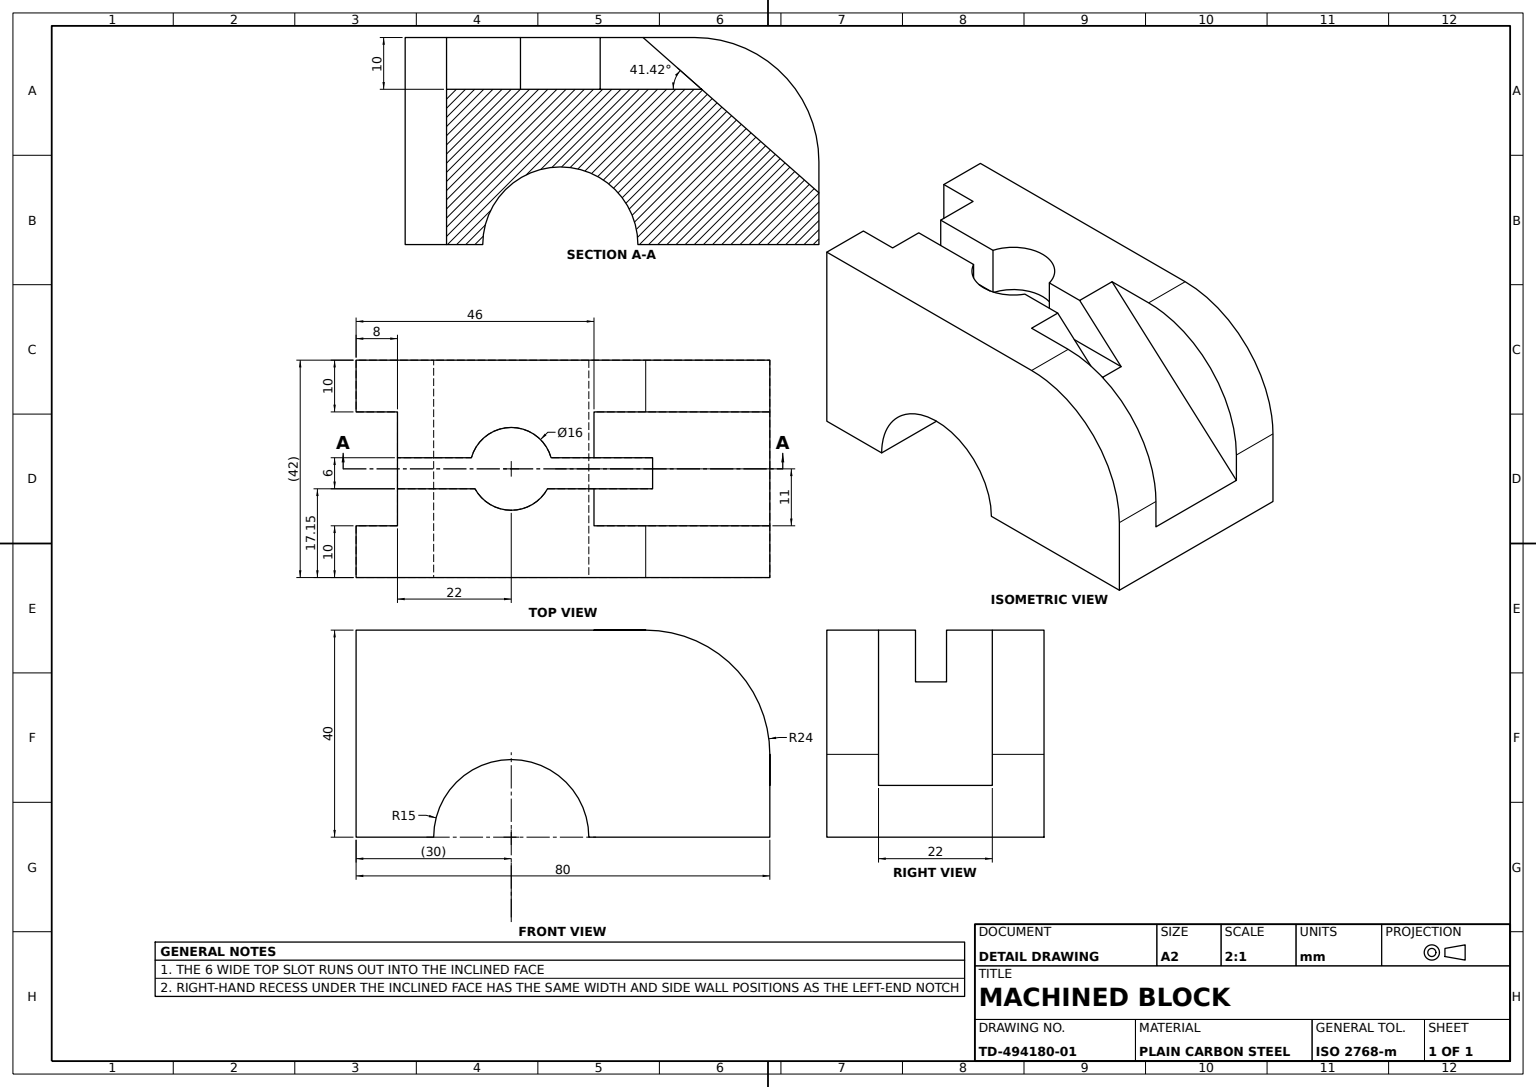
SolidWorks part; units mm, degrees
material "Plain Carbon Steel"
ref_plane "Front Plane" through (0, 0, 0) normal (0, 0, 1) x (1, 0, 0)
ref_plane "Top Plane" through (0, 0, 0) normal (0, 1, 0) x (1, 0, 0)
ref_plane "Right Plane" through (0, 0, 0) normal (1, 0, 0) x (0, 0, -1)
sketch "Bracket Profile Sketch" plane through (0, 0, 0) normal (0, 0, 1) x (1, 0, 0)
  line L0 (-40, 0) -> (40, 0)
  line L1 (-40, 0) -> (-40, 40)
  line L4 (-40, 40) -> (6, 40)
  line L5 (40, 0) -> (40, 10)
  line L6 (6, 40) -> (16, 40)
  line L7 (40, 16) -> (40, 10)
  arc A0 (16, 40) -> (40, 16) centre (16, 16) cw
  point P4 (0, 0)
  dimension "D5" = 24
  dimension "D1" = 80
  dimension "D2" = 40
  dimension "D3" = 10
  dimension "D4" = 46
extrude "Bracket Body" add sketch "Bracket Profile Sketch" against normal blind 42
sketch "Top Slot Sketch" plane through (0, 40, 0) normal (0, 1, 0) x (1, 0, 0)
  line L0 (-40, 23.1479) -> (-17.7063, 23.1479)
  line L1 (-40, 42) -> (-40, 0) construction
  line L2 (6, 23.1479) -> (6, 17.1479)
  line L3 (6, 17.1479) -> (-2.9885, 17.1479)
  line L4 (-40, 17.1479) -> (-40, 23.1479)
  line L5 (-2.2937, 23.1479) -> (6, 23.1479)
  line L6 (-17.0115, 17.1479) -> (-40, 17.1479)
  line L7 (16, 42) -> (16, 0) construction
  line L8 (16, 0) -> (-40, 0) construction
  arc A1 (-17.0115, 17.1479) -> (-2.9885, 17.1479) centre (-10, 21) ccw
  arc A2 (-2.2937, 23.1479) -> (-17.7063, 23.1479) centre (-10, 21) ccw
  point P6 (-40, 20.1479)
  dimension "D2" = 16
  dimension "D1" = 30
  dimension "D3" = 3
  dimension "D4" = 3
  dimension "D5" = 46
  dimension "D6" = 18.2937
  dimension "D7" = 17.1479
extrude "Top Slot Cut" cut sketch "Top Slot Sketch" against normal blind 10
sketch "Through Slot Sketch" plane through (0, 0, 0) normal (0, 0, 1) x (1, 0, 0)
  line L0 (-40, 40) -> (-40, 0) construction
  line L1 (16, 40) -> (-40, 40) construction
  line L2 (6, 40) -> (40, 10)
  line L4 (40, 0) -> (40, 16) construction
  line L5 (-40, 0) -> (40, 0) construction
  line L6 (40, 16) -> (40, 10)
  line L7 (16, 40) -> (6, 40)
  arc A0 (16, 40) -> (40, 16) centre (16, 16) cw
  dimension "D1" = 46
  dimension "D2" = 10
extrude "Through Slot 10mm" cut sketch "Through Slot Sketch" against normal blind 42
sketch "Slot Relief Sketch" plane through (6, 0, 0) normal (-1, 0, 0) x (0, 0, 1)
  line L0 (-23.1479, 40) -> (-23.1479, 30)
  line L1 (-23.1479, 30) -> (-17.1479, 30)
  line L2 (-17.1479, 30) -> (-17.1479, 40)
  line L3 (-17.1479, 40) -> (-23.1479, 40)
extrude "Slot Relief Cut" cut sketch "Slot Relief Sketch" against normal blind 42
sketch "Side Boss A Sketch" plane through (0, 0, 0) normal (0, 0, 1) x (1, 0, 0)
  line L1 (-40, 40) -> (40, 40)
  line L2 (-40, 40) -> (-40, 0)
  line L3 (-40, 0) -> (40, 0)
  line L4 (40, 40) -> (40, 0)
  line L5 (-40, 40) -> (40, 0) construction
  line L6 (-40, 0) -> (40, 40) construction
  point P4 (0, 20)
extrude "Side Boss A" add sketch "Side Boss A Sketch" against normal blind 10
sketch "Side Boss B Sketch" plane through (0, 0, -42) normal (0, 0, -1) x (-1, 0, 0)
  line L1 (40, 40) -> (-40, 40)
  line L2 (40, 40) -> (40, 0)
  line L3 (40, 0) -> (-40, 0)
  line L4 (-40, 40) -> (-40, 0)
  line L5 (40, 40) -> (-40, 0) construction
  line L6 (40, 0) -> (-40, 40) construction
  point P4 (0, 20)
extrude "Side Boss B" add sketch "Side Boss B Sketch" against normal blind 10
fillet "Corner Round R24" radius 24 2 edges at (40, 40, -37) (40, 40, -5)
sketch "Arch Cutout Sketch" plane through (0, 0, 0) normal (0, 0, 1) x (1, 0, 0)
  line L0 (-40, 0) -> (40, 0) construction
  line L1 (-25, 0) -> (5, 0)
  arc A0 (5, 0) -> (-25, 0) centre (-10, 0) ccw
  dimension "D1" = 30
  dimension "D2" = 30
extrude "Arch Cutout" cut sketch "Arch Cutout Sketch" against normal blind 42
sketch "Notch Sketch" plane through (0, 40, 0) normal (0, 1, 0) x (1, 0, 0)
  line L0 (-40, 32) -> (-32, 32)
  line L1 (-40, 42) -> (-40, 23.1479) construction
  line L2 (-32, 32) -> (-32, 10)
  line L3 (-32, 10) -> (-40, 10)
  line L4 (-40, 17.1479) -> (-40, 0) construction
  line L5 (-40, 10) -> (-40, 32)
  line L6 (16, 42) -> (-40, 42) construction
  line L7 (16, 0) -> (-40, 0) construction
  dimension "D1" = 10
  dimension "D2" = 10
  dimension "D3" = 8
extrude "Notch Cut" cut sketch "Notch Sketch" against normal blind 42
